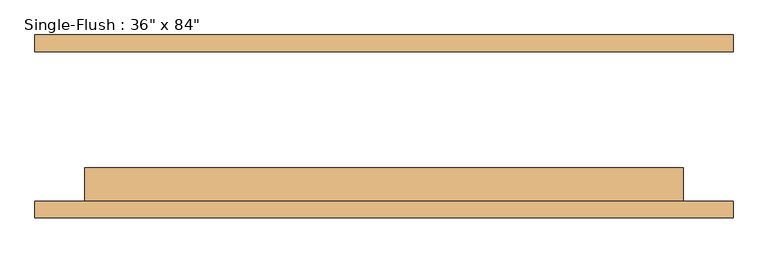
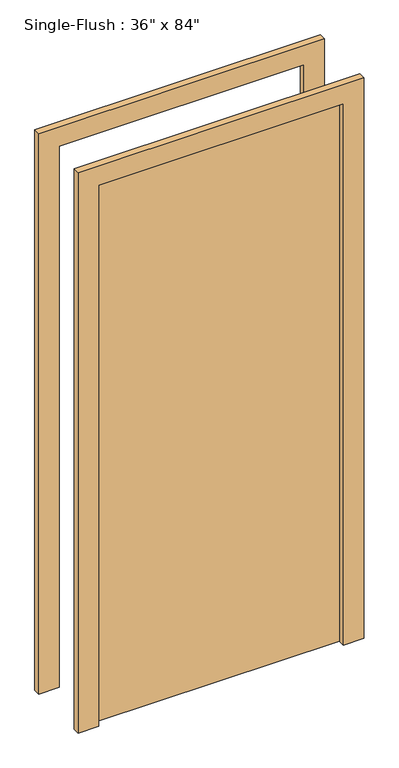
"""IFC4 building model written with IfcOpenShell, lengths in millimetres: door geometry."""

from ifc_helpers import new_model, si_unit, frame, origin, origin_with_axes, place, context, project, spatial, polyline, outline, extrude, source, transform, mapped, element, save


def door_a90ba1ad(model_context):
    return source(origin(), model_context, "Body", "SweptSolid", [
        extrude(outline(polyline([(2209.8, -533.4), (0.0, -533.4), (0.0, -457.2), (2133.6, -457.2), (2133.6, 457.2), (0.0, 457.2), (0.0, 533.4), (2209.8, 533.4), (2209.8, -533.4)])), frame((0.0, -139.7, 0.0), z_axis=(0.0, 1.0, 0.0), x_axis=(0.0, 0.0, 1.0)), (0.0, 0.0, 1.0), 25.4),
        extrude(outline(polyline([(2209.8, 533.4), (2209.8, -533.4), (0.0, -533.4), (0.0, -457.2), (2133.6, -457.2), (2133.6, 457.2), (0.0, 457.2), (0.0, 533.4), (2209.8, 533.4)])), frame((0.0, 114.3, 0.0), z_axis=(0.0, 1.0, 0.0), x_axis=(0.0, 0.0, 1.0)), (0.0, 0.0, 1.0), 25.4),
        extrude(outline(polyline([(457.2, -63.5), (457.2, -114.3), (-457.2, -114.3), (-457.2, -63.5), (457.2, -63.5)])), origin_with_axes(), (0.0, 0.0, 1.0), 2133.6),
    ])


if __name__ == "__main__":
    model = new_model("IFC4")
    model_context = context("Model", 3, world=origin())
    ifc_project = project(units=[si_unit("LENGTHUNIT", "METRE", prefix="MILLI")], contexts=[model_context])
    site = spatial("IfcSite", under=ifc_project)
    building = spatial("IfcBuilding", under=site)
    placement = place(None, origin())
    door_shape = door_a90ba1ad(model_context)
    element("IfcDoor", 1, ObjectType="Single-Flush : 36\" x 84\"", at=placement, inside=building, context=model_context, shape_type="MappedRepresentation", body=[
        mapped(door_shape, transform((0.0, 0.0, 0.0), x_axis=(1.0, 0.0, 0.0), y_axis=(0.0, 1.0, 0.0), z_axis=(0.0, 0.0, 1.0))),
    ])
    save(model, "model.ifc")

# Revit data of these elements
# Type "Single-Flush : 36\" x 84\""
#   Type Mark = "1"
#   Construction Type Id = "MDOOR"
#   Assembly Code = "C1020"
#   Analytic Construction = "Metal"
#   Thickness = 0' - 2"
#   Heat Transfer Coefficient (U) = 0.651978 BTU/(h·ft²·°F)
#   Height = 7' - 0"
#   Trim Projection Ext = 0' - 1"
#   Trim Projection Int = 0' - 1"
#   Trim Width = 0' - 3"
#   Width = 3' - 0"
#   Define Thermal Properties by = 1
#   Door Material = Door - Panel
#   Frame Material = Door - Frame
#   Visual Light Transmittance = 0
#   Solar Heat Gain Coefficient = 0
#   Function = (empty or 0)
#   Wall Closure = (empty or 0)
# Element 1 (IfcDoor, "Single-Flush : 36\" x 84\"")
#   Materials on its faces: "Door - Frame", "Door - Panel"
# Materials
#   "Door - Panel": class "Wood", colour RGB 210 159 95, transparency 0
#   "Door - Frame": colour RGB 118 70 51, transparency 0
